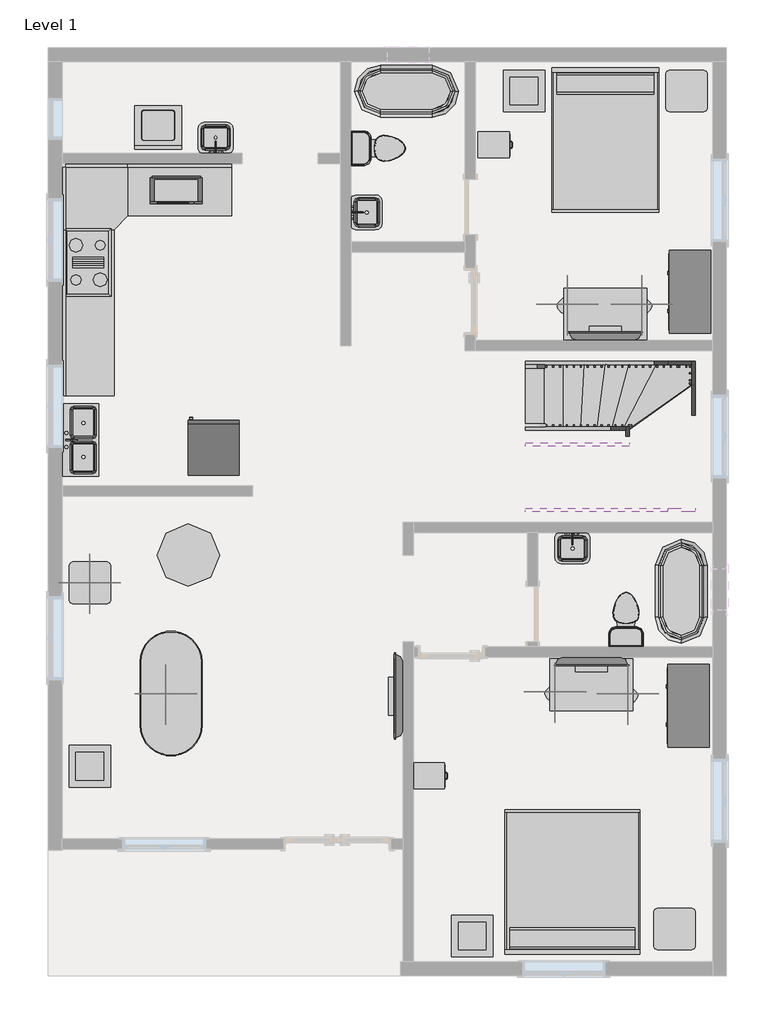
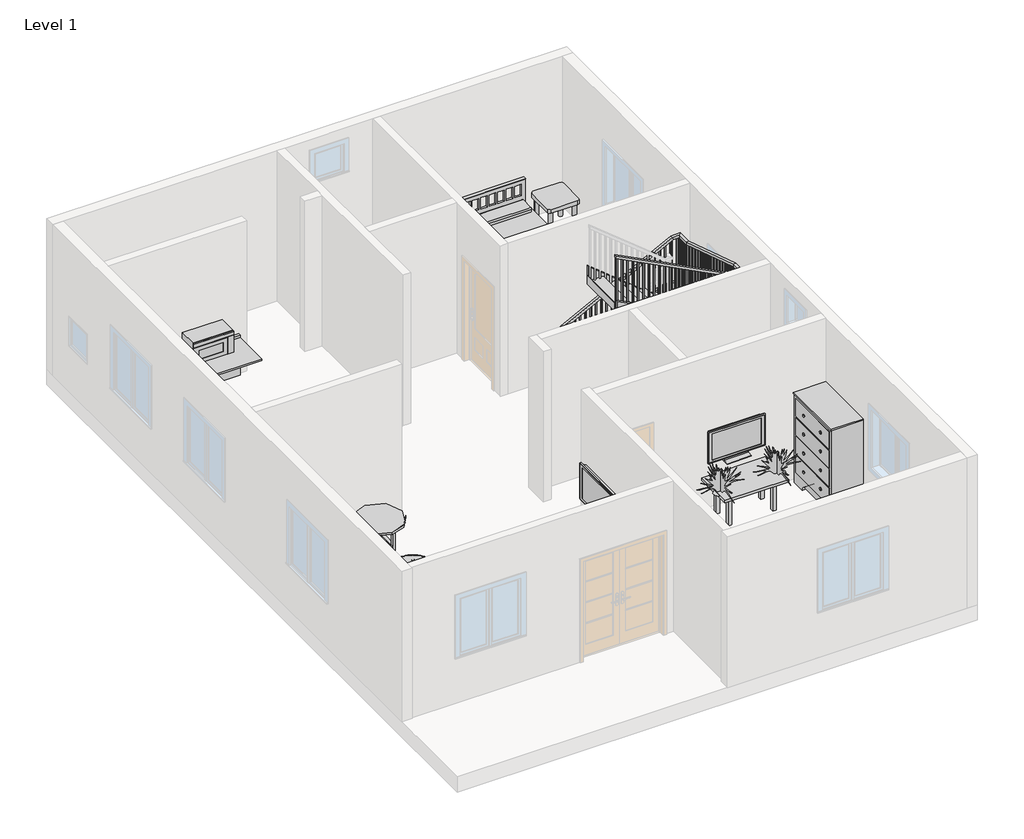
# One storey, part 2 of 2: 20 furniture elements, 11 flow terminals, 8 members, 6 geographic elements, 4 proxies, 1 railing, 1 stair flight.
# Revit data of these elements (continued)
# Type "Handrail - Rectangular" (continued)
#   built-in parameter 1008604 = 0.166667 (stored number, unit not read)
#   built-in parameter 1008603 = 0.166667 (stored number, unit not read)
#   Railing Height = 3' - 0"
#   built-in parameter 1008630 = 2
#   built-in parameter 1008610 = 2
#   built-in parameter 1008618 = Baluster - Square : 3/4"
# Element 1 (IfcBuildingElementProxy, "Cook Top-4 Unit : 36\" x 20\"")
#   Phase Created = New Construction
#   Materials on its faces: "Steel, Chrome Plated", "Steel, Polished"
# Element 2 (IfcBuildingElementProxy, "Microwave : 30\" x 16\" x 18\"")
#   Phase Created = New Construction
#   Materials on its faces: "Laminate, Ivory, Matte", "Glass"
# Element 3 (IfcBuildingElementProxy, "Refrigerator : 30\" x 32\" RH")
#   Phase Created = New Construction
#   Materials on its faces: "Steel, Paint Finish, Ivory, Glossy", "Steel, Chrome Plated"
# Element 4 (IfcBuildingElementProxy, "Washer : 27\" x 25\" x 35\"")
#   Phase Created = New Construction
#   Materials on its faces: "Steel, Paint Finish, Ivory, Matte"
# Element 5 (IfcFlowTerminal, "Floor Drain - Round : 5\" Strainer - 2\" Drain")
#   Mark = "1"
#   Phase Created = New Construction
# Element 6 (IfcFlowTerminal, "Floor Drain - Round : 5\" Strainer - 2\" Drain")
#   Mark = "7"
#   Phase Created = New Construction
# Element 7 (IfcFlowTerminal, "Floor Drain - Round : 5\" Strainer - 2\" Drain")
#   Mark = "11"
#   Phase Created = New Construction
# Element 8 (IfcFlowTerminal, "Sink Kitchen-Double : 42\" x 21\"")
#   Mark = "3"
#   Phase Created = New Construction
#   Materials on its faces: "Steel, Polished"
# Element 9 (IfcFlowTerminal, "Sink Vanity-Square : 20\" x 18\"")
#   Mark = "2"
#   Phase Created = New Construction
#   Materials on its faces: "Porcelain, Linen", "Steel, Polished"
# Element 10 (IfcFlowTerminal, "Sink Vanity-Square : 20\" x 18\"")
#   Mark = "4"
#   Phase Created = New Construction
#   Materials on its faces: "Porcelain, Linen", "Steel, Polished"
# Element 11 (IfcFlowTerminal, "Sink Vanity-Square : 20\" x 18\"")
#   Mark = "9"
#   Phase Created = New Construction
#   Materials on its faces: "Porcelain, Linen", "Steel, Polished"
# Element 12 (IfcFlowTerminal, "Toilet-Domestic-3D : Toilet-Domestic-3D")
#   Mark = "6"
#   Phase Created = New Construction
#   Materials on its faces: "Porcelain, Linen", "Laminate, Linen, Matte"
# Element 13 (IfcFlowTerminal, "Toilet-Domestic-3D : Toilet-Domestic-3D")
#   Mark = "10"
#   Phase Created = New Construction
#   Materials on its faces: "Porcelain, Linen", "Laminate, Linen, Matte"
# Element 14 (IfcFlowTerminal, "Tub-Free Standing-3D : 30\" x 60\"")
#   Mark = "5"
#   Phase Created = New Construction
#   Materials on its faces: "Porcelain, Ivory"
# Element 15 (IfcFlowTerminal, "Tub-Free Standing-3D : 30\" x 60\"")
#   Mark = "8"
#   Phase Created = New Construction
#   Materials on its faces: "Porcelain, Ivory"
# Element 16 (IfcFurniture, "Bed-Shaker : King 78\" x 83\"")
#   Phase Created = New Construction
#   Materials on its faces: "Birch", "Softwood, Lumber"
# Element 17 (IfcFurniture, "Bed-Shaker : Queen 62\" x 83\"")
#   Phase Created = New Construction
#   Materials on its faces: "Birch", "Softwood, Lumber"
# Elements 18, 19 (IfcFurniture, "Cabinet-File 2 Drawer : 15\" x 18\"")
#   Phase Created = New Construction
#   Materials on its faces: "Steel, Chrome Plated", "Steel, Paint Finish, Ivory, Glossy"
# Elements 20, 21 (IfcFurniture, "Dresser : 48\" x 72\" x 24\"")
#   Phase Created = New Construction
#   Materials on its faces: "Laminate, Ivory, Matte", "Cherry", "Wood - Teak"
# Elements 22, 23 (IfcFurniture, "TV - Flat Screen : 42\"")
#   Stand = yes
#   Phase Created = New Construction
#   Materials on its faces: "TV - Black", "TV - Glass", "TV - Screen"
# Element 24 (IfcFurniture, "TV - Flat Screen : 50\"")
#   Stand = yes
#   Phase Created = New Construction
#   Materials on its faces: "TV - Black", "TV - Glass", "TV - Screen"
# Elements 25, 26, 27 (IfcFurniture, "Table-Coffee : 24\" x 24\" x 24\"")
#   Phase Created = New Construction
#   Materials on its faces: "Glass - Clear, Grey"
# Element 28 (IfcFurniture, "Table-Dining Oval : 36\" x 72\"")
#   Phase Created = New Construction
#   Materials on its faces: "Steel, Chrome Plated", "Glass - Clear, Grey"
# Element 29 (IfcFurniture, "Table-Dining Round w Chairs : 36\" Diameter")
#   Phase Created = New Construction
#   Materials on its faces: "Pine", "Laminate, Linen, Matte"
# Elements 30, 31, 32 (IfcFurniture, "Table-End : 24\" x 24\"")
#   Phase Created = New Construction
#   Materials on its faces: "Laminate, Ivory, Matte", "Birch"
# Elements 33, 34 (IfcFurniture, "Table-Rectangular : 72\" x 30\"")
#   Phase Created = New Construction
#   Materials on its faces: "Birch"
# Element 35 (IfcFurniture, "Work Station Cubicle : 96\" x 96\"")
#   Phase Created = New Construction
#   Materials on its faces: "Textile - Light Gray", "Laminate, Ivory, Matte"
# Elements 36, 37, 38, 39, 40, 41 (IfcGeographicElement, "RPC Plant - Tropical : Agave - 1.5'")
#   Phase Created = New Construction
# Elements 42, 43, 44, 45, 46, 47, 48, 49 (IfcMember, "Stringer - 2\" Width")
#   Phase Created = New Construction
# Element 50 (IfcRailing, "Handrail - Rectangular")
#   Phase Created = New Construction
# Element 51 (IfcStairFlight, "2\" Tread 1\" Nosing 1/4\" Riser")
#   Phase Created = New Construction
# Materials
#   "Steel, Chrome Plated": class "Metal", colour RGB 17 17 17, transparency 0, Description = "Chromiuim plated steel", Cost = 0
#   "Steel, Polished": class "Metal", colour RGB 57 57 57, transparency 0, Description = "Polished steel", Cost = 0
#   "Laminate, Ivory, Matte": class "Plastic", colour RGB 247 247 239, transparency 0, Description = "Plastic Laminate - Ivory, Matte", Cost = 0
#   "Steel, Paint Finish, Ivory, Glossy": class "Metal", colour RGB 247 247 239, transparency 0, Description = "Steel, paint finish, ivory, glossy", Cost = 0
#   "Steel, Paint Finish, Ivory, Matte": class "Metal", colour RGB 247 247 239, transparency 0, Description = "Steel, paint finish, ivory, matte", Cost = 0
#   "Porcelain, Linen": class "Ceramic", colour RGB 249 239 230, transparency 0, Description = "Porcelain, linen", Cost = 0
#   "Laminate, Linen, Matte": class "Plastic", colour RGB 249 239 230, transparency 0, Description = "Plastic Laminate - Linen, Matte", Cost = 0
#   "Porcelain, Ivory": class "Ceramic", colour RGB 247 247 239, transparency 0, Description = "Porcelain, ivory", Cost = 0
#   "Birch": class "Wood", colour RGB 210 159 95, transparency 0, Description = "Betula Alleghaniensis", Cost = 0
#   "Softwood, Lumber": class "Wood", colour RGB 223 192 134, transparency 0, Description = "Pinus Echinata", Cost = 0
#   "Wood - Teak": class "Wood", colour RGB 145 112 90, transparency 0
#   "Cherry": class "Wood", colour RGB 226 177 128, transparency 0, Description = "Prunus Serotina", Cost = 0
#   "Glass - Clear, Grey": class "Glass", colour RGB 252 255 255, transparency 0.64
#   "Pine": class "Wood", colour RGB 223 192 134, transparency 0, Description = "Pinus Echinata", Cost = 0
#   "Textile - Light Gray": class "Fabric", colour RGB 204 204 204, transparency 0
#   "Glass": class "Glass", colour RGB 0 128 192, transparency 0.75, Description = "Soda Lime Glass", Cost = 0
#   "TV - Black": colour RGB 49 49 49, transparency 0
#   "TV - Glass": colour RGB 157 157 157, transparency 0.9
#   "TV - Screen": colour RGB 0 0 0, transparency 0
